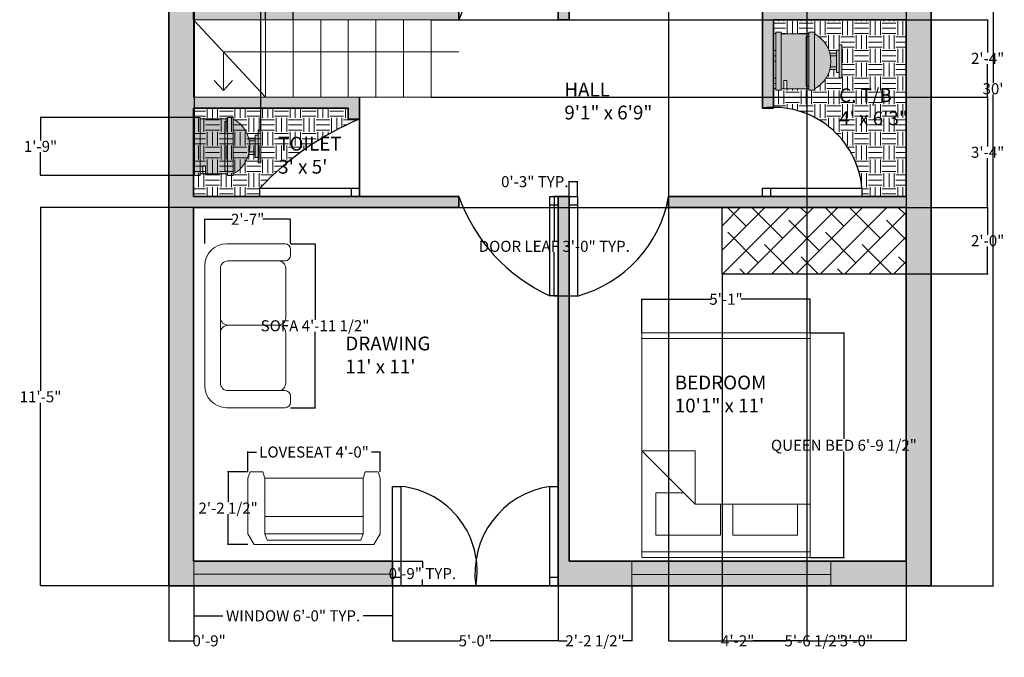
# Model space of a CAD drawing. Units: inches. Extents: x 490 to 851, y 299 to 716.
# Tile 1 of 3: x 493 to 849, y 299 to 530. Entities that reach past the tile are written whole.
import ezdxf

# ---------------------------------------------------------------- set-up
doc = ezdxf.new("R2010")
doc.units = ezdxf.units.IN
doc.header["$MEASUREMENT"] = 0
for name, color, linetype, lineweight in [('A-ANNO-DIMS', 2, 'Continuous', 18), ('A-AREA-IDEN', 7, 'Continuous', 25), ('A-DOOR', 3, 'Continuous', 25), ('A-FLOR-CASE', 40, 'Continuous', 25), ('A-FLOR-CASE-PATT', 9, 'Continuous', 13), ('A-FLOR-FIXT', 8, 'Continuous', 18), ('A-FLOR-FIXT-PATT', 9, 'Continuous', 13), ('A-FLOR-PATT', 4, 'Continuous', 13), ('A-FURN', 40, 'Continuous', 18), ('A-GLAZ', 4, 'Continuous', 18), ('A-GLAZ-PATT', 4, 'Continuous', 13), ('A-WALL', 7, 'Continuous', 35), ('A-WALL-PATT', 1, 'Continuous', 13), ('beds', 40, 'Continuous', 18), ('stairs', 82, 'Continuous', 18)]:
    doc.layers.add(name, color=color, linetype=linetype, lineweight=lineweight)
doc.styles.get("Standard").update_dxf_attribs({"font": 'arial.ttf'})
doc.dimstyles.get("Standard").update_dxf_attribs({"dimtxt": 4, "dimasz": 0.18, "dimexe": 0.18, "dimexo": 0.0625, "dimgap": 0.09, "dimtad": 0, "dimtih": 1, "dimtoh": 1, "dimdec": 0, "dimrnd": 6, "dimzin": 0, "dimdsep": 46, "dimlunit": 3, "dimtxsty": 'Standard', "dimcen": 0.09, "dimadec": 0, "dimazin": 0, "dimtfac": 1, "dimtdec": 0, "dimtofl": 0, "dimtmove": 0, "dimatfit": 3, "dimfxl": 1, "dimtolj": 1, "dimtzin": 0, "dimarcsym": 0})

# ---------------------------------------------------------------- blocks, each defined once
blk = doc.blocks.new('QUEEN-00')
for p, q in [((-0.8475, -0.7751), (-0.8475, 0.7489)), ((0.6511, 0.7489), (0.6511, -0.2925)), ((1.0829, 0.7489), (1.0829, -0.7751)), ((0.9305, 0.6346), (0.6511, 0.6346)), ((0.9305, 0.0504), (0.9305, 0.6346)), ((0.6511, 0.0504), (0.9305, 0.0504)), ((0.9305, -0.0639), (0.6511, -0.0639)), ((0.9305, -0.6481), (0.9305, -0.0639)), ((0.1685, -0.7751), (0.6511, -0.2925)), ((0.1685, -0.2925), (0.1685, -0.7751)), ((0.6511, -0.2925), (0.1685, -0.2925)), ((0.5495, -0.3941), (0.5495, -0.6481)), ((0.5495, -0.6481), (0.9305, -0.6481))]:
    blk.add_line(p, q)
blk.add_lwpolyline([(-0.8983, -0.7751), (-0.8983, 0.7489), (1.1337, 0.7489), (1.1337, -0.7751)], close=True)
blk = doc.blocks.new('A$C6BA70F2F')
for p, q in [((0.2, 0.7857), (1.3031, 0.7857)), ((0.2263, 0.6431), (1.2768, 0.6431)), ((0, 0.05), (0, 0.5857)), ((0.1563, 0.05), (0.1563, 0.5731)), ((0.7563, 0.5835), (0.7563, 0.1071)), ((0.7563, 0.1131), (0.7563, 0.5731)), ((1.3468, 0.05), (1.3468, 0.5731)), ((1.5031, 0.05), (1.5031, 0.5857)), ((0.6863, 0.0431), (0.2263, 0.0431)), ((1.2768, 0.0431), (0.8263, 0.0431)), ((0.1063, 0), (0.05, 0)), ((1.3968, 0), (1.4531, 0))]:
    blk.add_line(p, q)
for centre, radius, start, end in [((0.2, 0.5857), 0.2, 90, 180), ((1.3031, 0.5857), 0.2, 0, 90), ((0.2263, 0.5731), 0.07, 90, 180), ((0.6863, 0.5731), 0.07, 0, 90), ((0.8263, 0.5731), 0.07, 90, 180), ((1.2768, 0.5731), 0.07, 0, 90), ((0.2263, 0.1131), 0.07, 180, 270), ((0.6863, 0.1131), 0.07, 270, 0), ((0.8263, 0.1131), 0.07, 180, 270), ((1.2768, 0.1131), 0.07, 270, 0), ((0.05, 0.05), 0.05, 180, 270), ((0.1063, 0.05), 0.05, 270, 0), ((1.3968, 0.05), 0.05, 180, 270), ((1.4531, 0.05), 0.05, 270, 0)]:
    blk.add_arc(centre, radius, start, end)
blk = doc.blocks.new('A$C61201922')
for p, q in [((0, 0.737), (0.076, 0.864)), ((0.076, 0.864), (1.499, 0.864)), ((1.499, 0.864), (1.575, 0.737)), ((0, 0.076), (0, 0.737)), ((0.203, 0.737), (0.229, 0.813)), ((0.203, 0.076), (0.203, 0.737)), ((1.372, 0.737), (0.203, 0.737)), ((0.229, 0.813), (1.346, 0.813)), ((1.346, 0.813), (1.372, 0.737)), ((1.372, 0.737), (1.372, 0.076)), ((1.575, 0.737), (1.575, 0.076)), ((1.372, 0.533), (0.203, 0.533)), ((0.025, 0), (0, 0.076)), ((0.178, 0), (0.025, 0)), ((0.203, 0.076), (0.178, 0)), ((1.372, 0.076), (0.203, 0.076)), ((1.397, 0), (1.372, 0.076)), ((1.549, 0), (1.397, 0)), ((1.575, 0.076), (1.549, 0))]:
    blk.add_line(p, q)
blk = doc.blocks.new('Toilet - Imperial')
for p, q in [((-10, 22), (-10, 12)), ((10, 12), (10, 22)), ((-10, 21), (-7, 21)), ((-7, 20), (-10, 20)), ((-7, 21), (-7, 20)), ((10.5, 12), (-10.5, 12)), ((-10.5, 10), (-10.5, 12)), ((9, 13), (-9, 13)), ((-9, 13), (-9, 12)), ((9, 12), (9, 13)), ((10.5, 12), (10.5, 10)), ((10.5, 10), (-10.5, 10)), ((-3, 4.4065), (-3, 2)), ((-2, 2), (-2, 4.1658)), ((2, 4.1658), (2, 2)), ((3, 2), (3, 4.4065)), ((4, 2), (-4, 2)), ((-4, 2), (-4, 1)), ((4, 1), (4, 2))]:
    blk.add_line(p, q)
for points in [[(10.5, 22), (10.5, 24), (-10.5, 24), (-10.5, 22)], [(6, 0), (6, 1), (-6, 1), (-6, 0)]]:
    blk.add_lwpolyline(points, close=True)
blk.add_arc((0, 15.3333), 11.3333, 208.0725, 331.9275)
blk = doc.blocks.new('*D103')
at = {"layer": 'A-ANNO-DIMS', "color": 0, "lineweight": -2, "transparency": 16777216}
for p, q in [((822.75, 684.96), (845.33, 684.96)), ((845.15, 684.78), (845.15, 507.09)), ((845.15, 325.14), (845.15, 502.82)), ((822.75, 324.96), (845.33, 324.96))]:
    blk.add_line(p, q, dxfattribs=at)
at = {"layer": 'A-ANNO-DIMS', "color": 0, "transparency": 16777216}
for points in [[(845.12, 684.78), (845.18, 684.78), (845.15, 684.96)], [(845.12, 325.14), (845.18, 325.14), (845.15, 324.96)]]:
    blk.add_solid(points, dxfattribs=at)
at = {"layer": 'Defpoints', "color": 0, "transparency": 16777216}
for p in [(822.69, 684.96), (822.69, 324.96), (845.15, 324.96)]:
    blk.add_point(p, dxfattribs=at)
at = {"layer": 'A-ANNO-DIMS', "color": 0, "transparency": 16777216, "insert": (845.15, 504.96), "char_height": 4, "attachment_point": 5}
blk.add_mtext("\\A1;30'", dxfattribs=at)
blk = doc.blocks.new('DOOR-LEAF-36IN')
blk.add_line((3, 3), (0, 3))
blk.add_lwpolyline([(0, 0), (0, 36), (3, 36), (3, 0)], close=True)
blk = doc.blocks.new('WINDOW-72IN')
blk.add_line((0, 4.23), (72, 4.23))
blk.add_lwpolyline([(0, 0), (0, 9), (72, 9), (72, 0)], close=True)
blk = doc.blocks.new('*D106')
at = {"layer": 'A-ANNO-DIMS', "color": 0, "lineweight": -2, "transparency": 16777216}
for p, q in [((691.62, 465.92), (686.1, 465.92)), ((686.28, 465.74), (686.28, 450.08)), ((686.28, 430.1), (686.28, 445.76)), ((691.62, 429.92), (686.1, 429.92))]:
    blk.add_line(p, q, dxfattribs=at)
at = {"layer": 'A-ANNO-DIMS', "color": 0, "transparency": 16777216}
for points in [[(686.25, 465.74), (686.31, 465.74), (686.28, 465.92)], [(686.25, 430.1), (686.31, 430.1), (686.28, 429.92)]]:
    blk.add_solid(points, dxfattribs=at)
at = {"layer": 'Defpoints', "color": 0, "transparency": 16777216}
for p in [(691.68, 465.92), (686.28, 429.92), (691.68, 429.92)]:
    blk.add_point(p, dxfattribs=at)
at = {"layer": 'A-ANNO-DIMS', "color": 0, "transparency": 16777216, "insert": (686.28, 447.92), "char_height": 4, "attachment_point": 5}
blk.add_mtext('\\A1;DOOR LEAF 3\'-0" TYP.', dxfattribs=at)
blk = doc.blocks.new('*D107')
at = {"layer": 'A-ANNO-DIMS', "color": 0, "lineweight": -2, "transparency": 16777216}
for p, q in [((691.68, 471.32), (691.5, 471.32)), ((691.68, 465.98), (691.68, 471.5)), ((694.5, 471.32), (691.86, 471.32)), ((694.68, 465.98), (694.68, 471.5))]:
    blk.add_line(p, q, dxfattribs=at)
at = {"layer": 'A-ANNO-DIMS', "color": 0, "transparency": 16777216}
for points in [[(691.86, 471.35), (691.86, 471.29), (691.68, 471.32)], [(694.5, 471.35), (694.5, 471.29), (694.68, 471.32)]]:
    blk.add_solid(points, dxfattribs=at)
at = {"layer": 'Defpoints', "color": 0, "transparency": 16777216}
for p in [(691.68, 471.32), (691.68, 465.92), (694.68, 465.92)]:
    blk.add_point(p, dxfattribs=at)
at = {"layer": 'A-ANNO-DIMS', "color": 0, "transparency": 16777216, "insert": (679.22, 471.32), "char_height": 4, "attachment_point": 5}
blk.add_mtext('\\A1;0\'-3" TYP.', dxfattribs=at)
blk = doc.blocks.new('*D108')
at = {"layer": 'A-ANNO-DIMS', "color": 0, "lineweight": -2, "transparency": 16777216}
for p, q in [((555.71, 324.89), (555.71, 313.98)), ((627.71, 324.89), (627.71, 313.98)), ((555.89, 314.16), (566.31, 314.16)), ((627.53, 314.16), (617.11, 314.16))]:
    blk.add_line(p, q, dxfattribs=at)
at = {"layer": 'A-ANNO-DIMS', "color": 0, "transparency": 16777216}
for points in [[(555.89, 314.19), (555.89, 314.13), (555.71, 314.16)], [(627.53, 314.19), (627.53, 314.13), (627.71, 314.16)]]:
    blk.add_solid(points, dxfattribs=at)
at = {"layer": 'Defpoints', "color": 0, "transparency": 16777216}
for p in [(555.71, 324.96), (627.71, 324.96), (627.71, 314.16)]:
    blk.add_point(p, dxfattribs=at)
at = {"layer": 'A-ANNO-DIMS', "color": 0, "transparency": 16777216, "insert": (591.71, 314.16), "char_height": 4, "attachment_point": 5}
blk.add_mtext('\\A1;WINDOW 6\'-0" TYP.', dxfattribs=at)
blk = doc.blocks.new('*D109')
at = {"layer": 'A-ANNO-DIMS', "color": 0, "lineweight": -2, "transparency": 16777216}
for p, q in [((627.77, 333.96), (638.69, 333.96)), ((638.51, 333.78), (638.51, 331.59)), ((627.77, 324.96), (638.69, 324.96)), ((638.51, 325.14), (638.51, 327.32))]:
    blk.add_line(p, q, dxfattribs=at)
at = {"layer": 'A-ANNO-DIMS', "color": 0, "transparency": 16777216}
for points in [[(638.48, 333.78), (638.54, 333.78), (638.51, 333.96)], [(638.48, 325.14), (638.54, 325.14), (638.51, 324.96)]]:
    blk.add_solid(points, dxfattribs=at)
at = {"layer": 'Defpoints', "color": 0, "transparency": 16777216}
for p in [(627.71, 333.96), (638.51, 333.96), (627.71, 324.96)]:
    blk.add_point(p, dxfattribs=at)
at = {"layer": 'A-ANNO-DIMS', "color": 0, "transparency": 16777216, "insert": (638.51, 329.46), "char_height": 4, "attachment_point": 5}
blk.add_mtext('\\A1;0\'-9" TYP.', dxfattribs=at)
blk = doc.blocks.new('*D110')
at = {"layer": 'A-ANNO-DIMS', "color": 0, "lineweight": -2, "transparency": 16777216}
for p, q in [((779.01, 416.57), (791.33, 416.57)), ((791.15, 416.39), (791.15, 378.19)), ((791.15, 335.42), (791.15, 373.63)), ((779.01, 335.24), (791.33, 335.24))]:
    blk.add_line(p, q, dxfattribs=at)
at = {"layer": 'A-ANNO-DIMS', "color": 0, "transparency": 16777216}
for points in [[(791.12, 416.39), (791.18, 416.39), (791.15, 416.57)], [(791.12, 335.42), (791.18, 335.42), (791.15, 335.24)]]:
    blk.add_solid(points, dxfattribs=at)
at = {"layer": 'Defpoints', "color": 0, "transparency": 16777216}
for p in [(778.95, 416.57), (778.95, 335.24), (791.15, 335.24)]:
    blk.add_point(p, dxfattribs=at)
at = {"layer": 'A-ANNO-DIMS', "color": 0, "transparency": 16777216, "insert": (791.15, 375.91), "char_height": 4, "attachment_point": 5}
blk.add_mtext('\\A1;QUEEN BED 6\'-9 1/2"', dxfattribs=at)
blk = doc.blocks.new('*D111')
at = {"layer": 'A-ANNO-DIMS', "color": 0, "lineweight": -2, "transparency": 16777216}
for p, q in [((717.95, 416.64), (717.95, 428.95)), ((718.13, 428.77), (743.04, 428.77)), ((778.77, 428.77), (753.86, 428.77)), ((778.95, 416.64), (778.95, 428.95))]:
    blk.add_line(p, q, dxfattribs=at)
at = {"layer": 'A-ANNO-DIMS', "color": 0, "transparency": 16777216}
for points in [[(718.13, 428.8), (718.13, 428.74), (717.95, 428.77)], [(778.77, 428.8), (778.77, 428.74), (778.95, 428.77)]]:
    blk.add_solid(points, dxfattribs=at)
at = {"layer": 'Defpoints', "color": 0, "transparency": 16777216}
for p in [(778.95, 428.77), (717.95, 416.57), (778.95, 416.57)]:
    blk.add_point(p, dxfattribs=at)
at = {"layer": 'A-ANNO-DIMS', "color": 0, "transparency": 16777216, "insert": (748.45, 428.77), "char_height": 4, "attachment_point": 5}
blk.add_mtext('\\A1;5\'-1"', dxfattribs=at)
blk = doc.blocks.new('*D118')
at = {"layer": 'A-ANNO-DIMS', "color": 0, "lineweight": -2, "transparency": 16777216}
for p, q in [((590.81, 448.82), (599.83, 448.82)), ((599.65, 448.64), (599.65, 421.32)), ((599.65, 389.68), (599.65, 417)), ((590.81, 389.5), (599.83, 389.5))]:
    blk.add_line(p, q, dxfattribs=at)
at = {"layer": 'A-ANNO-DIMS', "color": 0, "transparency": 16777216}
for points in [[(599.62, 448.64), (599.68, 448.64), (599.65, 448.82)], [(599.62, 389.68), (599.68, 389.68), (599.65, 389.5)]]:
    blk.add_solid(points, dxfattribs=at)
at = {"layer": 'Defpoints', "color": 0, "transparency": 16777216}
for p in [(590.75, 448.82), (599.65, 448.82), (590.75, 389.5)]:
    blk.add_point(p, dxfattribs=at)
at = {"layer": 'A-ANNO-DIMS', "color": 0, "transparency": 16777216, "insert": (599.65, 419.16), "char_height": 4, "attachment_point": 5}
blk.add_mtext('\\A1;SOFA 4\'-11 1/2"', dxfattribs=at)
blk = doc.blocks.new('*D119')
at = {"layer": 'A-ANNO-DIMS', "color": 0, "lineweight": -2, "transparency": 16777216}
for p, q in [((559.75, 448.88), (559.75, 457.9)), ((559.93, 457.72), (569.81, 457.72)), ((590.57, 457.72), (580.69, 457.72)), ((590.75, 448.88), (590.75, 457.9))]:
    blk.add_line(p, q, dxfattribs=at)
at = {"layer": 'A-ANNO-DIMS', "color": 0, "transparency": 16777216}
for points in [[(559.93, 457.75), (559.93, 457.69), (559.75, 457.72)], [(590.57, 457.75), (590.57, 457.69), (590.75, 457.72)]]:
    blk.add_solid(points, dxfattribs=at)
at = {"layer": 'Defpoints', "color": 0, "transparency": 16777216}
for p in [(559.75, 457.72), (559.75, 448.82), (590.75, 448.82)]:
    blk.add_point(p, dxfattribs=at)
at = {"layer": 'A-ANNO-DIMS', "color": 0, "transparency": 16777216, "insert": (575.25, 457.72), "char_height": 4, "attachment_point": 5}
blk.add_mtext('\\A1;2\'-7"', dxfattribs=at)
blk = doc.blocks.new('*D120')
at = {"layer": 'A-ANNO-DIMS', "color": 0, "lineweight": -2, "transparency": 16777216}
for p, q in [((575.35, 366.33), (575.35, 373.63)), ((575.53, 373.45), (578.45, 373.45)), ((623.05, 373.45), (620.14, 373.45)), ((623.23, 366.33), (623.23, 373.63))]:
    blk.add_line(p, q, dxfattribs=at)
at = {"layer": 'A-ANNO-DIMS', "color": 0, "transparency": 16777216}
for points in [[(575.53, 373.48), (575.53, 373.42), (575.35, 373.45)], [(623.05, 373.48), (623.05, 373.42), (623.23, 373.45)]]:
    blk.add_solid(points, dxfattribs=at)
at = {"layer": 'Defpoints', "color": 0, "transparency": 16777216}
for p in [(575.35, 373.45), (575.35, 366.27), (623.23, 366.27)]:
    blk.add_point(p, dxfattribs=at)
at = {"layer": 'A-ANNO-DIMS', "color": 0, "transparency": 16777216, "insert": (599.29, 373.45), "char_height": 4, "attachment_point": 5}
blk.add_mtext('\\A1;LOVESEAT 4\'-0"', dxfattribs=at)
blk = doc.blocks.new('*D121')
at = {"layer": 'A-ANNO-DIMS', "color": 0, "lineweight": -2, "transparency": 16777216}
for p, q in [((575.29, 366.27), (567.99, 366.27)), ((568.17, 366.09), (568.17, 355.3)), ((568.17, 340.19), (568.17, 350.98)), ((575.29, 340.01), (567.99, 340.01))]:
    blk.add_line(p, q, dxfattribs=at)
at = {"layer": 'A-ANNO-DIMS', "color": 0, "transparency": 16777216}
for points in [[(568.14, 366.09), (568.2, 366.09), (568.17, 366.27)], [(568.14, 340.19), (568.2, 340.19), (568.17, 340.01)]]:
    blk.add_solid(points, dxfattribs=at)
at = {"layer": 'Defpoints', "color": 0, "transparency": 16777216}
for p in [(575.35, 366.27), (568.17, 340.01), (575.35, 340.01)]:
    blk.add_point(p, dxfattribs=at)
at = {"layer": 'A-ANNO-DIMS', "color": 0, "transparency": 16777216, "insert": (568.17, 353.14), "char_height": 4, "attachment_point": 5}
blk.add_mtext('\\A1;2\'-2 1/2"', dxfattribs=at)
blk = doc.blocks.new('*D126')
at = {"layer": 'A-ANNO-DIMS', "color": 0, "lineweight": -2, "transparency": 16777216}
for p, q in [((747.06, 437.89), (747.06, 304.93)), ((813.69, 437.89), (813.69, 304.93)), ((747.24, 305.11), (770.31, 305.11)), ((813.51, 305.11), (790.44, 305.11))]:
    blk.add_line(p, q, dxfattribs=at)
at = {"layer": 'A-ANNO-DIMS', "color": 0, "transparency": 16777216}
for points in [[(747.24, 305.14), (747.24, 305.08), (747.06, 305.11)], [(813.51, 305.14), (813.51, 305.08), (813.69, 305.11)]]:
    blk.add_solid(points, dxfattribs=at)
at = {"layer": 'Defpoints', "color": 0, "transparency": 16777216}
for p in [(747.06, 437.96), (813.69, 437.96), (813.69, 305.11)]:
    blk.add_point(p, dxfattribs=at)
at = {"layer": 'A-ANNO-DIMS', "color": 0, "transparency": 16777216, "insert": (780.38, 305.11), "char_height": 4, "attachment_point": 5}
blk.add_mtext('\\A1;5\'-6 1/2"', dxfattribs=at)
blk = doc.blocks.new('*D127')
at = {"layer": 'A-ANNO-DIMS', "color": 0, "lineweight": -2, "transparency": 16777216}
for p, q in [((813.75, 461.96), (843.38, 461.96)), ((843.2, 461.78), (843.2, 452.09)), ((843.2, 438.14), (843.2, 447.82)), ((813.75, 437.96), (843.38, 437.96))]:
    blk.add_line(p, q, dxfattribs=at)
at = {"layer": 'A-ANNO-DIMS', "color": 0, "transparency": 16777216}
for points in [[(843.17, 461.78), (843.23, 461.78), (843.2, 461.96)], [(843.17, 438.14), (843.23, 438.14), (843.2, 437.96)]]:
    blk.add_solid(points, dxfattribs=at)
at = {"layer": 'Defpoints', "color": 0, "transparency": 16777216}
for p in [(813.69, 461.96), (843.2, 461.96), (813.69, 437.96)]:
    blk.add_point(p, dxfattribs=at)
at = {"layer": 'A-ANNO-DIMS', "color": 0, "transparency": 16777216, "insert": (843.2, 449.96), "char_height": 4, "attachment_point": 5}
blk.add_mtext('\\A1;2\'-0"', dxfattribs=at)
blk = doc.blocks.new('*D128')
at = {"layer": 'A-ANNO-DIMS', "color": 0, "lineweight": -2, "transparency": 16777216}
for p, q in [((555.63, 461.96), (500.07, 461.96)), ((500.25, 461.78), (500.25, 395.59)), ((500.25, 325.14), (500.25, 391.32)), ((546.63, 324.96), (500.07, 324.96))]:
    blk.add_line(p, q, dxfattribs=at)
at = {"layer": 'A-ANNO-DIMS', "color": 0, "transparency": 16777216}
for points in [[(500.22, 461.78), (500.28, 461.78), (500.25, 461.96)], [(500.22, 325.14), (500.28, 325.14), (500.25, 324.96)]]:
    blk.add_solid(points, dxfattribs=at)
at = {"layer": 'Defpoints', "color": 0, "transparency": 16777216}
for p in [(500.25, 461.96), (555.69, 461.96), (546.69, 324.96)]:
    blk.add_point(p, dxfattribs=at)
at = {"layer": 'A-ANNO-DIMS', "color": 0, "transparency": 16777216, "insert": (500.25, 393.46), "char_height": 4, "attachment_point": 5}
blk.add_mtext('\\A1;11\'-5"', dxfattribs=at)
blk = doc.blocks.new('*D129')
at = {"layer": 'A-ANNO-DIMS', "color": 0, "lineweight": -2, "transparency": 16777216}
for p, q in [((641.75, 529.96), (843.38, 529.96)), ((843.2, 529.78), (843.2, 518.06)), ((843.2, 502.14), (843.2, 513.86)), ((641.75, 501.96), (843.38, 501.96))]:
    blk.add_line(p, q, dxfattribs=at)
at = {"layer": 'A-ANNO-DIMS', "color": 0, "transparency": 16777216}
for points in [[(843.17, 529.78), (843.23, 529.78), (843.2, 529.96)], [(843.17, 502.14), (843.23, 502.14), (843.2, 501.96)]]:
    blk.add_solid(points, dxfattribs=at)
at = {"layer": 'Defpoints', "color": 0, "transparency": 16777216}
for p in [(641.69, 529.96), (843.2, 529.96), (641.69, 501.96)]:
    blk.add_point(p, dxfattribs=at)
at = {"layer": 'A-ANNO-DIMS', "color": 0, "transparency": 16777216, "insert": (843.2, 515.96), "char_height": 4, "attachment_point": 5}
blk.add_mtext('\\A1;2\'-4"', dxfattribs=at)
blk = doc.blocks.new('*D130')
at = {"layer": 'A-ANNO-DIMS', "color": 0, "lineweight": -2, "transparency": 16777216}
for p, q in [((641.75, 501.96), (843.38, 501.96)), ((843.2, 501.78), (843.2, 484.09)), ((843.2, 462.14), (843.2, 479.82)), ((651.75, 461.96), (843.38, 461.96))]:
    blk.add_line(p, q, dxfattribs=at)
at = {"layer": 'A-ANNO-DIMS', "color": 0, "transparency": 16777216}
for points in [[(843.17, 501.78), (843.23, 501.78), (843.2, 501.96)], [(843.17, 462.14), (843.23, 462.14), (843.2, 461.96)]]:
    blk.add_solid(points, dxfattribs=at)
at = {"layer": 'Defpoints', "color": 0, "transparency": 16777216}
for p in [(641.69, 501.96), (843.2, 501.96), (651.69, 461.96)]:
    blk.add_point(p, dxfattribs=at)
at = {"layer": 'A-ANNO-DIMS', "color": 0, "transparency": 16777216, "insert": (843.2, 481.96), "char_height": 4, "attachment_point": 5}
blk.add_mtext('\\A1;3\'-4"', dxfattribs=at)
blk = doc.blocks.new('*D131')
at = {"layer": 'A-ANNO-DIMS', "color": 0, "lineweight": -2, "transparency": 16777216}
for p, q in [((555.69, 530.02), (555.69, 704.89)), ((555.87, 704.71), (563.25, 704.71)), ((581.51, 704.71), (574.13, 704.71)), ((581.69, 530.02), (581.69, 704.89))]:
    blk.add_line(p, q, dxfattribs=at)
at = {"layer": 'A-ANNO-DIMS', "color": 0, "transparency": 16777216}
for points in [[(555.87, 704.74), (555.87, 704.68), (555.69, 704.71)], [(581.51, 704.74), (581.51, 704.68), (581.69, 704.71)]]:
    blk.add_solid(points, dxfattribs=at)
at = {"layer": 'Defpoints', "color": 0, "transparency": 16777216}
for p in [(581.69, 704.71), (555.69, 529.96), (581.69, 529.96)]:
    blk.add_point(p, dxfattribs=at)
at = {"layer": 'A-ANNO-DIMS', "color": 0, "transparency": 16777216, "insert": (568.69, 704.71), "char_height": 4, "attachment_point": 5}
blk.add_mtext('\\A1;2\'-2"', dxfattribs=at)
blk = doc.blocks.new('*D132')
at = {"layer": 'A-ANNO-DIMS', "color": 0, "lineweight": -2, "transparency": 16777216}
for p, q in [((581.69, 530.02), (581.69, 704.89)), ((581.87, 704.71), (591.51, 704.71)), ((591.69, 530.02), (591.69, 704.89)), ((591.69, 704.71), (591.87, 704.71))]:
    blk.add_line(p, q, dxfattribs=at)
at = {"layer": 'A-ANNO-DIMS', "color": 0, "transparency": 16777216}
for points in [[(581.87, 704.74), (581.87, 704.68), (581.69, 704.71)], [(591.51, 704.74), (591.51, 704.68), (591.69, 704.71)]]:
    blk.add_solid(points, dxfattribs=at)
at = {"layer": 'Defpoints', "color": 0, "transparency": 16777216}
for p in [(591.69, 704.71), (581.69, 529.96), (591.69, 529.96)]:
    blk.add_point(p, dxfattribs=at)
at = {"layer": 'A-ANNO-DIMS', "color": 0, "transparency": 16777216, "insert": (598.83, 704.71), "char_height": 4, "attachment_point": 5}
blk.add_mtext('\\A1;0\'-10"', dxfattribs=at)
blk = doc.blocks.new('*D133')
at = {"layer": 'A-ANNO-DIMS', "color": 0, "lineweight": -2, "transparency": 16777216}
for p, q in [((546.69, 324.89), (546.69, 304.93)), ((555.71, 324.89), (555.71, 304.93)), ((546.87, 305.11), (555.53, 305.11)), ((555.71, 305.11), (555.89, 305.11))]:
    blk.add_line(p, q, dxfattribs=at)
at = {"layer": 'A-ANNO-DIMS', "color": 0, "transparency": 16777216}
for points in [[(546.87, 305.14), (546.87, 305.08), (546.69, 305.11)], [(555.53, 305.14), (555.53, 305.08), (555.71, 305.11)]]:
    blk.add_solid(points, dxfattribs=at)
at = {"layer": 'Defpoints', "color": 0, "transparency": 16777216}
for p in [(546.69, 324.96), (555.71, 324.96), (555.71, 305.11)]:
    blk.add_point(p, dxfattribs=at)
at = {"layer": 'A-ANNO-DIMS', "color": 0, "transparency": 16777216, "insert": (561.29, 305.11), "char_height": 4, "attachment_point": 5}
blk.add_mtext('\\A1;0\'-9"', dxfattribs=at)
blk = doc.blocks.new('*D134')
at = {"layer": 'A-ANNO-DIMS', "color": 0, "lineweight": -2, "transparency": 16777216}
for p, q in [((627.69, 324.89), (627.69, 304.93)), ((687.69, 324.89), (687.69, 304.93)), ((627.87, 305.11), (652.28, 305.11)), ((687.51, 305.11), (663.09, 305.11))]:
    blk.add_line(p, q, dxfattribs=at)
at = {"layer": 'A-ANNO-DIMS', "color": 0, "transparency": 16777216}
for points in [[(627.87, 305.14), (627.87, 305.08), (627.69, 305.11)], [(687.51, 305.14), (687.51, 305.08), (687.69, 305.11)]]:
    blk.add_solid(points, dxfattribs=at)
at = {"layer": 'Defpoints', "color": 0, "transparency": 16777216}
for p in [(627.69, 324.96), (687.69, 324.96), (687.69, 305.11)]:
    blk.add_point(p, dxfattribs=at)
at = {"layer": 'A-ANNO-DIMS', "color": 0, "transparency": 16777216, "insert": (657.69, 305.11), "char_height": 4, "attachment_point": 5}
blk.add_mtext('\\A1;5\'-0"', dxfattribs=at)
blk = doc.blocks.new('*D135')
at = {"layer": 'A-ANNO-DIMS', "color": 0, "lineweight": -2, "transparency": 16777216}
for p, q in [((687.69, 324.89), (687.69, 304.93)), ((714.39, 324.8), (714.39, 304.93)), ((687.87, 305.11), (690.94, 305.11)), ((714.21, 305.11), (711.14, 305.11))]:
    blk.add_line(p, q, dxfattribs=at)
at = {"layer": 'A-ANNO-DIMS', "color": 0, "transparency": 16777216}
for points in [[(687.87, 305.14), (687.87, 305.08), (687.69, 305.11)], [(714.21, 305.14), (714.21, 305.08), (714.39, 305.11)]]:
    blk.add_solid(points, dxfattribs=at)
at = {"layer": 'Defpoints', "color": 0, "transparency": 16777216}
for p in [(687.69, 324.96), (714.39, 324.86), (714.39, 305.11)]:
    blk.add_point(p, dxfattribs=at)
at = {"layer": 'A-ANNO-DIMS', "color": 0, "transparency": 16777216, "insert": (701.04, 305.11), "char_height": 4, "attachment_point": 5}
blk.add_mtext('\\A1;2\'-2 1/2"', dxfattribs=at)
blk = doc.blocks.new('*D136')
at = {"layer": 'A-ANNO-DIMS', "color": 0, "lineweight": -2, "transparency": 16777216}
for p, q in [((556, 494.66), (556, 704.89)), ((556.18, 704.71), (562.56, 704.71)), ((579.82, 704.71), (573.44, 704.71)), ((580, 490.16), (580, 704.89))]:
    blk.add_line(p, q, dxfattribs=at)
at = {"layer": 'A-ANNO-DIMS', "color": 0, "transparency": 16777216}
for points in [[(556.18, 704.74), (556.18, 704.68), (556, 704.71)], [(579.82, 704.74), (579.82, 704.68), (580, 704.71)]]:
    blk.add_solid(points, dxfattribs=at)
at = {"layer": 'Defpoints', "color": 0, "transparency": 16777216}
for p in [(580, 704.71), (556, 494.6), (580, 490.1)]:
    blk.add_point(p, dxfattribs=at)
at = {"layer": 'A-ANNO-DIMS', "color": 0, "transparency": 16777216, "insert": (568, 704.71), "char_height": 4, "attachment_point": 5}
blk.add_mtext('\\A1;2\'-0"', dxfattribs=at)
blk = doc.blocks.new('*D137')
at = {"layer": 'A-ANNO-DIMS', "color": 0, "lineweight": -2, "transparency": 16777216}
for p, q in [((555.94, 494.6), (500.07, 494.6)), ((500.25, 494.42), (500.25, 486.23)), ((500.25, 473.78), (500.25, 481.97)), ((555.94, 473.6), (500.07, 473.6))]:
    blk.add_line(p, q, dxfattribs=at)
at = {"layer": 'A-ANNO-DIMS', "color": 0, "transparency": 16777216}
for points in [[(500.22, 494.42), (500.28, 494.42), (500.25, 494.6)], [(500.22, 473.78), (500.28, 473.78), (500.25, 473.6)]]:
    blk.add_solid(points, dxfattribs=at)
at = {"layer": 'Defpoints', "color": 0, "transparency": 16777216}
for p in [(500.25, 494.6), (556, 494.6), (556, 473.6)]:
    blk.add_point(p, dxfattribs=at)
at = {"layer": 'A-ANNO-DIMS', "color": 0, "transparency": 16777216, "insert": (500.25, 484.1), "char_height": 4, "attachment_point": 5}
blk.add_mtext('\\A1;1\'-9"', dxfattribs=at)
blk = doc.blocks.new('*D138')
at = {"layer": 'A-ANNO-DIMS', "color": 0, "lineweight": -2, "transparency": 16777216}
for p, q in [((777.69, 600.89), (777.69, 304.93)), ((813.69, 600.89), (813.69, 304.93)), ((777.87, 305.11), (790.28, 305.11)), ((813.51, 305.11), (801.09, 305.11))]:
    blk.add_line(p, q, dxfattribs=at)
at = {"layer": 'A-ANNO-DIMS', "color": 0, "transparency": 16777216}
for points in [[(777.87, 305.14), (777.87, 305.08), (777.69, 305.11)], [(813.51, 305.14), (813.51, 305.08), (813.69, 305.11)]]:
    blk.add_solid(points, dxfattribs=at)
at = {"layer": 'Defpoints', "color": 0, "transparency": 16777216}
for p in [(777.69, 600.96), (813.69, 600.96), (813.69, 305.11)]:
    blk.add_point(p, dxfattribs=at)
at = {"layer": 'A-ANNO-DIMS', "color": 0, "transparency": 16777216, "insert": (795.69, 305.11), "char_height": 4, "attachment_point": 5}
blk.add_mtext('\\A1;3\'-0"', dxfattribs=at)
blk = doc.blocks.new('*D143')
at = {"layer": 'A-ANNO-DIMS', "color": 0, "lineweight": -2, "transparency": 16777216}
for p, q in [((727.69, 560.89), (727.69, 304.93)), ((777.69, 560.89), (777.69, 304.93)), ((727.87, 305.11), (747.2, 305.11)), ((777.51, 305.11), (758.17, 305.11))]:
    blk.add_line(p, q, dxfattribs=at)
at = {"layer": 'A-ANNO-DIMS', "color": 0, "transparency": 16777216}
for points in [[(727.87, 305.14), (727.87, 305.08), (727.69, 305.11)], [(777.51, 305.14), (777.51, 305.08), (777.69, 305.11)]]:
    blk.add_solid(points, dxfattribs=at)
at = {"layer": 'Defpoints', "color": 0, "transparency": 16777216}
for p in [(727.69, 560.96), (777.69, 560.96), (777.69, 305.11)]:
    blk.add_point(p, dxfattribs=at)
at = {"layer": 'A-ANNO-DIMS', "color": 0, "transparency": 16777216, "insert": (752.69, 305.11), "char_height": 4, "attachment_point": 5}
blk.add_mtext('\\A1;4\'-2"', dxfattribs=at)

msp = doc.modelspace()

# ---------------------------------------------------------------- hatches: boundary and pattern name
at = {"layer": 'A-FLOR-CASE-PATT'}
h = msp.add_hatch(dxfattribs=at)
h.set_pattern_fill('ANSI38', color=256, scale=50)
h.paths.add_polyline_path([(687.69, 675.96), (663.69, 675.96), (663.69, 583.46), (687.69, 583.46)])
h.paths.add_polyline_path([(813.69, 461.96), (747.06, 461.96), (747.06, 437.96), (813.69, 437.96)])
at = {"layer": 'A-FLOR-FIXT-PATT'}
h = msp.add_hatch(color=256, dxfattribs=at)
h.dxf.hatch_style = 1
h.paths.add_polyline_path([(567, 493.1), (568, 493.1), (568, 494.1), (558, 494.1), (558, 474.1), (559, 474.1), (559, 477.1), (560, 477.1), (560, 474.1), (568, 474.1), (568, 475.1), (567, 475.1)])
h.paths.add_polyline_path([(568, 493.1), (567, 493.1), (567, 475.1), (568, 475.1)], flags=17)
h.paths.add_polyline_path([(570, 494.6), (568, 494.6), (568, 473.6), (570, 473.6)])
h.paths.add_polyline_path([(570, 494.1), (570, 474.1, 0.600002)])
h.paths.add_polyline_path([(578, 486.1), (575.82, 486.1, -0.088933), (575.82, 482.1), (578, 482.1)])
h.paths.add_polyline_path([(579, 488.1), (578, 488.1), (578, 480.1), (579, 480.1)])
h.paths.add_polyline_path([(580, 490.1), (579, 490.1), (579, 478.1), (580, 478.1)])
h.paths.add_polyline_path([(578, 487.1), (575.6, 487.1, -0.022629), (575.82, 486.1), (578, 486.1)])
h.paths.add_polyline_path([(578, 482.1), (575.82, 482.1, -0.022629), (575.6, 481.1), (578, 481.1)])
h.paths.add_polyline_path([(558, 494.6), (556, 494.6), (556, 473.6), (558, 473.6)])
h.paths.add_polyline_path([(768.45, 525.39), (766.45, 525.39), (766.45, 504.39), (768.45, 504.39)])
h.paths.add_polyline_path([(777.45, 523.89), (778.45, 523.89), (778.45, 524.89), (768.45, 524.89), (768.45, 504.89), (769.45, 504.89), (769.45, 507.89), (770.45, 507.89), (770.45, 504.89), (778.45, 504.89), (778.45, 505.89), (777.45, 505.89)])
h.paths.add_polyline_path([(778.45, 523.89), (777.45, 523.89), (777.45, 505.89), (778.45, 505.89)], flags=17)
h.paths.add_polyline_path([(780.45, 525.39), (778.45, 525.39), (778.45, 504.39), (780.45, 504.39)])
h.paths.add_polyline_path([(780.45, 524.89), (780.45, 504.89, 0.600002)])
h.paths.add_polyline_path([(788.45, 516.89), (786.27, 516.89, -0.088933), (786.27, 512.89), (788.45, 512.89)])
h.paths.add_polyline_path([(789.45, 518.89), (788.45, 518.89), (788.45, 510.89), (789.45, 510.89)])
h.paths.add_polyline_path([(790.45, 520.89), (789.45, 520.89), (789.45, 508.89), (790.45, 508.89)])
h.paths.add_polyline_path([(788.45, 517.89), (786.05, 517.89, -0.022629), (786.27, 516.89), (788.45, 516.89)])
h.paths.add_polyline_path([(788.45, 512.89), (786.27, 512.89, -0.022629), (786.05, 511.89), (788.45, 511.89)])
at = {"layer": 'A-FLOR-PATT'}
h = msp.add_hatch(dxfattribs=at)
h.set_pattern_fill('EARTH', color=256, scale=20)
h.paths.add_polyline_path([(813.69, 529.96), (765.69, 529.96), (765.69, 498.21, -0.38858), (797.69, 468.96), (797.69, 465.96), (813.69, 465.96)])
h.paths.add_polyline_path([(790.45, 508.89), (789.45, 508.89), (789.45, 510.89), (788.45, 510.89), (788.45, 511.89), (786.05, 511.89, -0.206081), (780.45, 504.89), (780.45, 504.39), (778.45, 504.39), (778.45, 504.89), (768.45, 504.89), (768.45, 504.39), (766.45, 504.39), (766.45, 525.39), (768.45, 525.39), (768.45, 524.89), (778.45, 524.89), (778.45, 525.39), (780.45, 525.39), (780.45, 524.89, -0.206081), (786.05, 517.89), (788.45, 517.89), (788.45, 518.89), (789.45, 518.89), (789.45, 520.89), (790.45, 520.89)], flags=16)
h.paths.add_polyline_path([(787.84, 488.92), (814.78, 488.92), (814.78, 507.58), (787.84, 507.58)], flags=9)
h = msp.add_hatch(dxfattribs=at)
h.set_pattern_fill('EARTH', color=256, scale=20)
h.paths.add_polyline_path([(615.69, 493.96), (611.69, 493.96), (611.69, 497.96), (555.69, 497.96), (555.69, 465.96), (579.69, 465.96), (579.69, 468.96, -0.105572)])
at = {"layer": 'A-GLAZ-PATT'}
h = msp.add_hatch(color=256, dxfattribs=at)
h.dxf.hatch_style = 1
h.paths.add_polyline_path([(627.69, 333.96), (555.71, 333.96), (555.71, 329.19), (627.69, 329.19)])
h.paths.add_polyline_path([(627.69, 329.19), (555.71, 329.19), (555.71, 324.96), (627.69, 324.96)])
h.paths.add_polyline_path([(786.39, 333.86), (714.39, 333.86), (714.39, 329.09), (786.39, 329.09)])
h.paths.add_polyline_path([(786.39, 329.09), (714.39, 329.09), (714.39, 324.96), (786.39, 324.96)])
h.paths.add_polyline_path([(802.5, 533.96), (777.76, 533.96), (777.76, 532), (802.5, 532)])
h.paths.add_polyline_path([(802.5, 532), (777.76, 532), (777.76, 529.97), (802.5, 529.97)])
h.paths.add_polyline_path([(813.69, 562.98), (777.69, 562.98), (777.69, 560.96), (813.69, 560.96)])
h.paths.add_polyline_path([(813.69, 564.96), (777.69, 564.96), (777.69, 562.98), (813.69, 562.98)])
at = {"layer": 'A-WALL-PATT'}
h = msp.add_hatch(color=256, dxfattribs=at)
h.dxf.hatch_style = 1
h.paths.add_polyline_path([(555.69, 497.96), (611.69, 497.96), (611.69, 493.96), (615.69, 493.96), (615.69, 501.96), (555.69, 501.96), (555.69, 529.96), (651.69, 529.96), (651.69, 533.96), (555.69, 533.96), (555.69, 675.96), (813.69, 675.96), (813.69, 564.96), (813.69, 560.96), (813.69, 533.96), (802.5, 533.96), (802.5, 529.96), (813.69, 529.96), (813.69, 465.96), (727.69, 465.96), (727.69, 461.96), (813.69, 461.96), (813.69, 333.96), (786.39, 333.96), (786.39, 324.96), (822.69, 324.96), (822.69, 684.96), (546.69, 684.96), (546.69, 324.96), (555.71, 324.96), (555.71, 333.96), (555.69, 333.96), (555.69, 461.96), (651.69, 461.96), (651.69, 465.96), (555.69, 465.96)])
h.paths.add_polyline_path([(714.39, 333.96), (691.69, 333.96), (691.69, 429.92), (691.68, 429.92), (691.68, 465.96), (687.69, 465.96), (687.69, 429.96), (687.69, 361.01), (687.69, 361.01), (687.69, 324.96), (714.39, 324.96)], flags=17)
h.paths.add_polyline_path([(691.69, 675.96), (687.69, 675.96), (687.69, 529.96), (691.69, 529.96)], flags=17)
h.paths.add_polyline_path([(777.76, 533.96), (761.69, 533.96), (761.69, 497.96, -0.03124), (765.69, 498.21), (765.69, 529.96), (777.76, 529.96)], flags=17)
h.paths.add_polyline_path([(777.69, 564.96), (727.69, 564.96), (727.69, 560.96), (777.69, 560.96)], flags=17)

# ---------------------------------------------------------------- linework, layer by layer
at = {"layer": 'A-DOOR'}
for centre, radius, start, end in [((713.59, 506.39), 66.24, 115.8959, 159.1627), ((765.71, 466.1), 32.11, 5.0977, 97.1956), ((656.23, 397.16), 104.95, 112.7248, 136.8308), ((711.08, 487.28), 63.1, 199.7455, 245.2754), ((682.62, 474.1), 45.79, 285.2628, 349.7593), ((627.55, 330.39), 30.78, 349.9345, 84.1556), ((689.4, 329.5), 31.86, 98.4972, 188.1029)]:
    msp.add_arc(centre, radius, start, end, dxfattribs=at)
at = {"layer": 'A-FLOR-CASE'}
for q in [(747.06, 461.96), (813.69, 437.96)]:
    msp.add_line((747.06, 437.96), q, dxfattribs=at)
at = {"layer": 'A-WALL'}
for p, q in [((546.69, 684.96), (546.69, 324.96)), ((822.69, 324.96), (822.69, 684.96)), ((687.69, 675.96), (687.69, 529.96)), ((691.69, 675.96), (691.69, 529.96)), ((651.69, 533.96), (651.69, 529.96)), ((761.69, 497.96), (761.69, 533.96)), ((691.69, 529.96), (687.69, 529.96)), ((813.69, 529.96), (765.69, 529.96)), ((765.69, 497.96), (765.69, 529.96)), ((813.69, 465.96), (813.69, 529.96)), ((615.69, 501.96), (615.69, 465.96)), ((555.69, 497.96), (611.69, 497.96)), ((555.69, 497.96), (555.69, 465.96)), ((611.69, 497.96), (611.69, 493.96)), ((761.69, 497.96), (765.69, 497.96)), ((611.69, 493.96), (615.69, 493.96)), ((555.69, 465.96), (651.69, 465.96)), ((651.69, 465.96), (651.69, 461.96)), ((687.69, 465.96), (687.69, 324.96)), ((687.69, 465.96), (691.69, 465.96)), ((691.69, 465.96), (691.69, 333.96)), ((727.69, 465.96), (727.69, 461.96)), ((727.69, 465.96), (813.69, 465.96)), ((555.69, 461.96), (651.69, 461.96)), ((555.69, 461.96), (555.69, 333.96)), ((727.69, 461.96), (813.69, 461.96)), ((813.69, 333.96), (813.69, 461.96)), ((555.69, 333.96), (627.69, 333.96)), ((627.69, 333.96), (627.69, 324.96)), ((691.69, 333.96), (813.69, 333.96)), ((546.69, 324.96), (627.69, 324.96)), ((627.69, 324.96), (822.69, 324.96))]:
    msp.add_line(p, q, dxfattribs=at)
at = {"layer": 'stairs'}
for p, q in [((555.69, 529.96), (581.69, 501.96)), ((651.69, 529.96), (555.69, 529.96)), ((555.69, 529.96), (555.69, 501.96)), ((581.69, 529.96), (581.69, 501.96)), ((591.69, 529.96), (591.69, 501.96)), ((601.69, 529.96), (601.69, 501.96)), ((611.69, 529.96), (611.69, 501.96)), ((621.69, 529.96), (621.69, 501.96)), ((631.69, 529.96), (631.69, 501.96)), ((641.69, 529.96), (641.69, 501.96)), ((651.69, 518.37), (566.45, 518.37)), ((566.45, 518.37), (566.45, 504.36)), ((566.45, 504.36), (563.15, 507.97)), ((566.45, 504.36), (569.75, 507.97)), ((555.69, 501.96), (641.69, 501.96))]:
    msp.add_line(p, q, dxfattribs=at)

# ---------------------------------------------------------------- block references
at = {"layer": 'A-DOOR'}
for p, rotation in [((615.69, 465.96), 90.0000000000004), ((761.69, 468.96), 270.0000000000006), ((687.69, 465.96), 180), ((694.68, 465.92), 180)]:
    msp.add_blockref('DOOR-LEAF-36IN', p, dxfattribs=dict(at, rotation=rotation))
for p in [(627.69, 325.01), (684.69, 325.01)]:
    msp.add_blockref('DOOR-LEAF-36IN', p, dxfattribs=at)
at = {"layer": 'A-FLOR-FIXT', "rotation": 90}
for p in [(790.45, 514.89), (580, 484.1)]:
    msp.add_blockref('Toilet - Imperial', p, dxfattribs=at)
at = {"layer": 'A-FURN'}
for name, p, xscale, yscale, zscale, rotation in [('A$C6BA70F2F', (590.75, 389.5), 39.46233405548116, 39.46233405548116, 39.46233405548116, 90), ('A$C61201922', (623.23, 366.27), 30.40476369305528, 30.40476369305528, 30.40476369305528, 180)]:
    msp.add_blockref(name, p, dxfattribs=dict(at, xscale=xscale, yscale=yscale, zscale=zscale, rotation=rotation))
at = {"layer": 'A-GLAZ'}
for p in [(555.71, 324.96), (714.39, 324.86)]:
    msp.add_blockref('WINDOW-72IN', p, dxfattribs=at)
at = {"layer": 'beds', "xscale": 40.02481723340583, "yscale": 40.02481723340583, "zscale": 40.02481723340583, "rotation": 270}
msp.add_blockref('QUEEN-00', (748.97, 380.62), dxfattribs=at)

# ---------------------------------------------------------------- texts
at = {"layer": 'A-AREA-IDEN', "char_height": 5, "attachment_point": 1}
for s, insert in [('HALL\\P9\'1" x 6\'9"', (689.92, 507.18)), ('C. T/B\\P4\' x 6\'3"', (789.44, 505.09)), ("TOILET\\P3' x 5'", (586.31, 487.56)), ("DRAWING\\P11' x 11'", (610.63, 415.25)), ('BEDROOM\\P10\'1" x 11\'', (729.9, 401.11))]:
    msp.add_mtext_dynamic_manual_height_columns(s, width=54.9921, gutter_width=1, heights=[0], dxfattribs=dict(at, insert=insert))

# ---------------------------------------------------------------- dimensions: what is measured, and where the dimension line sits
at = {"layer": 'A-ANNO-DIMS'}
for base, p1, p2, picture, middle in [((581.69, 704.71), (555.69, 529.96), (581.69, 529.96), '*D131', (568.69, 704.71)), ((580, 704.71), (556, 494.6), (580, 490.1), '*D136', (568, 704.71)), ((591.69, 704.71), (581.69, 529.96), (591.69, 529.96), '*D132', (598.83, 704.71)), ((813.69, 305.11), (777.69, 600.96), (813.69, 600.96), '*D138', (795.69, 305.11)), ((777.69, 305.11), (727.69, 560.96), (777.69, 560.96), '*D143', (752.69, 305.11)), ((813.69, 305.11), (747.06, 437.96), (813.69, 437.96), '*D126', (780.38, 305.11)), ((778.95, 428.77), (717.95, 416.57), (778.95, 416.57), '*D111', (748.45, 428.77)), ((555.71, 305.11), (546.69, 324.96), (555.71, 324.96), '*D133', (561.29, 305.11)), ((687.69, 305.11), (627.69, 324.96), (687.69, 324.96), '*D134', (657.69, 305.11)), ((714.39, 305.11), (687.69, 324.96), (714.39, 324.86), '*D135', (701.04, 305.11))]:
    dim = msp.add_linear_dim(base=base, p1=p1, p2=p2, dimstyle='Standard', override={"dimdec": 1, "dimlfac": 1, "dimrnd": 0, "dimzin": 1, "dimdsep": 46, "dimlunit": 4, "dimfrac": 2}, dxfattribs=at)
    dim.commit()
    dim.dimension.update_dxf_attribs({"geometry": picture, "text_midpoint": middle})
for base, p1, p2, angle, override, picture, middle in [((845.15, 324.96), (822.69, 684.96), (822.69, 324.96), 90, {"dimclrd": 0, "dimclre": 0, "dimclrt": 0}, '*D103', (845.15, 504.96)), ((843.2, 529.96), (641.69, 501.96), (641.69, 529.96), 90, {"dimdec": 1, "dimlfac": 1, "dimrnd": 0, "dimzin": 1, "dimdsep": 46, "dimlunit": 4, "dimfrac": 2}, '*D129', (843.2, 515.96)), ((843.2, 501.96), (651.69, 461.96), (641.69, 501.96), 90, {"dimdec": 1, "dimlfac": 1, "dimrnd": 0, "dimzin": 1, "dimdsep": 46, "dimlunit": 4, "dimfrac": 2}, '*D130', (843.2, 481.96)), ((500.25, 494.6), (556, 473.6), (556, 494.6), 90, {"dimdec": 1, "dimlfac": 1, "dimrnd": 0, "dimzin": 1, "dimdsep": 46, "dimlunit": 4, "dimfrac": 2}, '*D137', (500.25, 484.1)), ((500.25, 461.96), (546.69, 324.96), (555.69, 461.96), 90, {"dimdec": 1, "dimlfac": 1, "dimrnd": 0, "dimzin": 1, "dimdsep": 46, "dimlunit": 4, "dimfrac": 2}, '*D128', (500.25, 393.46)), ((559.75, 457.72), (590.75, 448.82), (559.75, 448.82), 180, {"dimdec": 1, "dimlfac": 1, "dimrnd": 0, "dimzin": 1, "dimdsep": 46, "dimlunit": 4, "dimfrac": 2}, '*D119', (575.25, 457.72)), ((843.2, 461.96), (813.69, 437.96), (813.69, 461.96), 90, {"dimdec": 1, "dimlfac": 1, "dimrnd": 0, "dimzin": 1, "dimdsep": 46, "dimlunit": 4, "dimfrac": 2}, '*D127', (843.2, 449.96)), ((568.17, 340.01), (575.35, 366.27), (575.35, 340.01), 270, {"dimdec": 1, "dimlfac": 1, "dimrnd": 0, "dimzin": 1, "dimdsep": 46, "dimlunit": 4, "dimfrac": 2}, '*D121', (568.17, 353.14))]:
    dim = msp.add_linear_dim(base=base, p1=p1, p2=p2, angle=angle, dimstyle='Standard', override=override, dxfattribs=at)
    dim.commit()
    dim.dimension.update_dxf_attribs({"geometry": picture, "text_midpoint": middle})
for base, p1, p2, angle, text, picture, middle in [((691.68, 471.32), (694.68, 465.92), (691.68, 465.92), 180, '<> TYP.', '*D107', (679.22, 471.32)), ((686.28, 429.92), (691.68, 465.92), (691.68, 429.92), 270, 'DOOR LEAF <> TYP.', '*D106', (686.28, 447.92)), ((599.65, 448.82), (590.75, 389.5), (590.75, 448.82), 90, 'SOFA <>', '*D118', (599.65, 419.16)), ((791.15, 335.24), (778.95, 416.57), (778.95, 335.24), 270, 'QUEEN BED <>', '*D110', (791.15, 375.91)), ((575.35, 373.45), (623.23, 366.27), (575.35, 366.27), 180, 'LOVESEAT <>', '*D120', (599.29, 373.45)), ((638.51, 333.96), (627.71, 324.96), (627.71, 333.96), 90, '<> TYP.', '*D109', (638.51, 329.46))]:
    dim = msp.add_linear_dim(base=base, p1=p1, p2=p2, angle=angle, text=text, dimstyle='Standard', override={"dimdec": 1, "dimlfac": 1, "dimrnd": 0, "dimzin": 1, "dimdsep": 46, "dimlunit": 4, "dimfrac": 2}, dxfattribs=at)
    dim.commit()
    dim.dimension.update_dxf_attribs({"geometry": picture, "text_midpoint": middle})
dim = msp.add_linear_dim(base=(627.71, 314.16), p1=(555.71, 324.96), p2=(627.71, 324.96), text='WINDOW <> TYP.', dimstyle='Standard', override={"dimdec": 1, "dimlfac": 1, "dimrnd": 0, "dimzin": 1, "dimdsep": 46, "dimlunit": 4, "dimfrac": 2}, dxfattribs=at)
dim.commit()
dim.dimension.update_dxf_attribs({"geometry": '*D108', "text_midpoint": (591.71, 314.16)})

doc.saveas('drawing.dxf')
